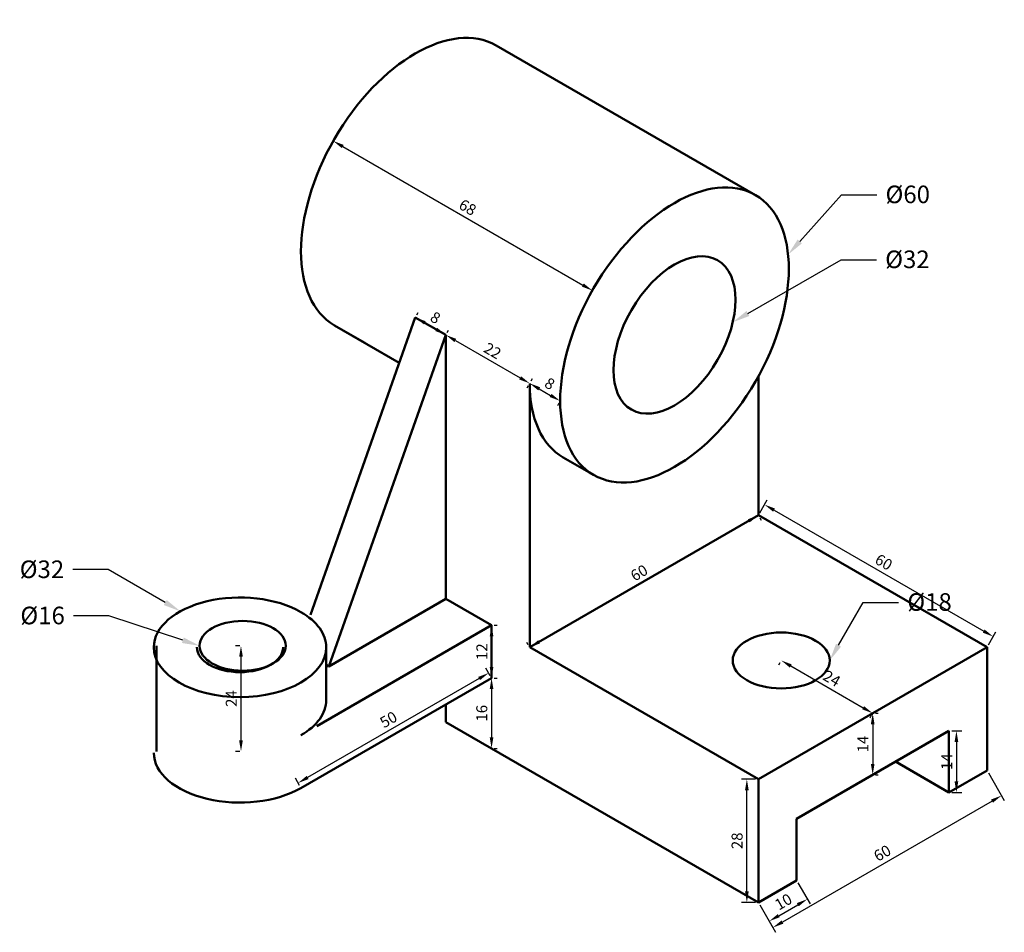
# Model space of a CAD drawing. Units: millimetres. Extents: x 3088 to 3311, y 622 to 830.
import ezdxf
from ezdxf import colors
from ezdxf.entities.mleader import LeaderData, LeaderLine
from ezdxf.math import Vec2, Vec3

# ---------------------------------------------------------------- set-up
doc = ezdxf.new("R2010")
doc.units = ezdxf.units.MM
for name, color, linetype, lineweight in [('M-DIMS', 2, 'Continuous', 25), ('M-OUTL', 7, 'Continuous', 50), ('M-TEXT', 3, 'Continuous', 25)]:
    doc.layers.add(name, color=color, linetype=linetype, lineweight=lineweight)
doc.styles.get("Standard").update_dxf_attribs({"font": 'arial.ttf'})
doc.dimstyles.new('ISO-25', dxfattribs={"dimtxt": 2.5, "dimasz": 2.5, "dimexe": 1.25, "dimexo": 0.625, "dimtad": 1, "dimtxsty": 'Standard', "dimcen": 2.5, "dimadec": 0, "dimazin": 0, "dimtfac": 1, "dimtmove": 0, "dimatfit": 3, "dimfxl": 1, "dimarcsym": 0})

# ---------------------------------------------------------------- blocks, each defined once
blk = doc.blocks.new('*D1')
at = {"layer": 'Defpoints', "color": 0, "transparency": 16777216}
for p in [(3264.1, 633.89), (3255.44, 628.89), (3266.57, 629.62)]:
    blk.add_point(p, dxfattribs=at)
at = {"layer": 'M-DIMS', "color": 0, "lineweight": -2, "transparency": 16777216}
for p, q in [((3264.41, 633.35), (3267.19, 628.53)), ((3255.75, 628.35), (3258.53, 623.53)), ((3260.07, 625.87), (3264.4, 628.37))]:
    blk.add_line(p, q, dxfattribs=at)
at = {"layer": 'M-DIMS', "color": 0, "transparency": 16777216}
for points in [[(3264.19, 628.73), (3264.61, 628.01), (3266.57, 629.62)], [(3259.86, 626.23), (3260.28, 625.51), (3257.91, 624.62)]]:
    blk.add_solid(points, dxfattribs=at)
at = {"layer": 'M-DIMS', "color": 0, "transparency": 16777216, "insert": (3261.29, 628.76), "char_height": 2.5, "attachment_point": 5, "rotation": 30}
blk.add_mtext('10', dxfattribs=at)
blk = doc.blocks.new('*D2')
at = {"layer": 'Defpoints', "color": 0, "transparency": 16777216}
for p in [(3281.42, 671.89), (3281.42, 657.89), (3281.42, 657.89)]:
    blk.add_point(p, dxfattribs=at)
at = {"layer": 'M-DIMS', "color": 0, "lineweight": -2, "transparency": 16777216}
for p, q in [((3282.05, 671.89), (3282.67, 671.89)), ((3281.42, 669.39), (3281.42, 660.39)), ((3282.05, 657.89), (3282.67, 657.89))]:
    blk.add_line(p, q, dxfattribs=at)
at = {"layer": 'M-DIMS', "color": 0, "transparency": 16777216}
for points in [[(3281, 669.39), (3281.84, 669.39), (3281.42, 671.89)], [(3281, 660.39), (3281.84, 660.39), (3281.42, 657.89)]]:
    blk.add_solid(points, dxfattribs=at)
at = {"layer": 'M-DIMS', "color": 0, "transparency": 16777216, "insert": (3279.54, 664.89), "char_height": 2.5, "attachment_point": 5, "rotation": 90}
blk.add_mtext('14', dxfattribs=at)
blk = doc.blocks.new('*D3')
at = {"layer": 'Defpoints', "color": 0, "transparency": 16777216}
for p in [(3307.4, 658.89), (3255.44, 628.89), (3258.74, 623.17)]:
    blk.add_point(p, dxfattribs=at)
at = {"layer": 'M-DIMS', "color": 0, "lineweight": -2, "transparency": 16777216}
for p, q in [((3307.71, 658.35), (3311.33, 652.09)), ((3308.54, 651.92), (3260.91, 624.42)), ((3255.75, 628.35), (3259.37, 622.09))]:
    blk.add_line(p, q, dxfattribs=at)
at = {"layer": 'M-DIMS', "color": 0, "transparency": 16777216}
for points in [[(3308.33, 652.28), (3308.75, 651.56), (3310.7, 653.17)], [(3260.7, 624.78), (3261.12, 624.06), (3258.74, 623.17)]]:
    blk.add_solid(points, dxfattribs=at)
at = {"layer": 'M-DIMS', "color": 0, "transparency": 16777216, "insert": (3283.77, 639.82), "char_height": 2.5, "attachment_point": 5, "rotation": 30}
blk.add_mtext('60', dxfattribs=at)
blk = doc.blocks.new('*D4')
at = {"layer": 'Defpoints', "color": 0, "transparency": 16777216}
for p in [(3252.83, 656.89), (3255.44, 656.89), (3255.44, 628.89)]:
    blk.add_point(p, dxfattribs=at)
at = {"layer": 'M-DIMS', "color": 0, "lineweight": -2, "transparency": 16777216}
for p, q in [((3254.81, 656.89), (3251.58, 656.89)), ((3252.83, 631.39), (3252.83, 654.39)), ((3254.81, 628.89), (3251.58, 628.89))]:
    blk.add_line(p, q, dxfattribs=at)
at = {"layer": 'M-DIMS', "color": 0, "transparency": 16777216}
for points in [[(3252.41, 654.39), (3253.25, 654.39), (3252.83, 656.89)], [(3252.41, 631.39), (3253.25, 631.39), (3252.83, 628.89)]]:
    blk.add_solid(points, dxfattribs=at)
at = {"layer": 'M-DIMS', "color": 0, "transparency": 16777216, "insert": (3250.93, 642.89), "char_height": 2.5, "attachment_point": 5, "rotation": 90}
blk.add_mtext('28', dxfattribs=at)
blk = doc.blocks.new('*D5')
at = {"layer": 'Defpoints', "color": 0, "transparency": 16777216}
for p in [(3194.82, 679.89), (3194.82, 663.89), (3194.82, 663.89)]:
    blk.add_point(p, dxfattribs=at)
at = {"layer": 'M-DIMS', "color": 0, "lineweight": -2, "transparency": 16777216}
for p, q in [((3195.44, 679.89), (3196.07, 679.89)), ((3194.82, 677.39), (3194.82, 666.39)), ((3195.44, 663.89), (3196.07, 663.89))]:
    blk.add_line(p, q, dxfattribs=at)
at = {"layer": 'M-DIMS', "color": 0, "transparency": 16777216}
for points in [[(3194.4, 677.39), (3195.23, 677.39), (3194.82, 679.89)], [(3194.4, 666.39), (3195.23, 666.39), (3194.82, 663.89)]]:
    blk.add_solid(points, dxfattribs=at)
at = {"layer": 'M-DIMS', "color": 0, "transparency": 16777216, "insert": (3192.92, 671.89), "char_height": 2.5, "attachment_point": 5, "rotation": 90}
blk.add_mtext('16', dxfattribs=at)
blk = doc.blocks.new('*D6')
at = {"layer": 'Defpoints', "color": 0, "transparency": 16777216}
for p in [(3194.82, 691.89), (3194.82, 679.89), (3194.82, 679.89)]:
    blk.add_point(p, dxfattribs=at)
at = {"layer": 'M-DIMS', "color": 0, "lineweight": -2, "transparency": 16777216}
for p, q in [((3195.44, 691.89), (3196.07, 691.89)), ((3194.82, 689.39), (3194.82, 682.39)), ((3195.44, 679.89), (3196.07, 679.89))]:
    blk.add_line(p, q, dxfattribs=at)
at = {"layer": 'M-DIMS', "color": 0, "transparency": 16777216}
for points in [[(3194.4, 689.39), (3195.23, 689.39), (3194.82, 691.89)], [(3194.4, 682.39), (3195.23, 682.39), (3194.82, 679.89)]]:
    blk.add_solid(points, dxfattribs=at)
at = {"layer": 'M-DIMS', "color": 0, "transparency": 16777216, "insert": (3192.94, 685.89), "char_height": 2.5, "attachment_point": 5, "rotation": 90}
blk.add_mtext('12', dxfattribs=at)
blk = doc.blocks.new('*D7')
at = {"layer": 'Defpoints', "color": 0, "transparency": 16777216}
for p in [(3255.44, 716.89), (3255.44, 716.89), (3203.48, 686.89)]:
    blk.add_point(p, dxfattribs=at)
at = {"layer": 'M-DIMS', "color": 0, "lineweight": -2, "transparency": 16777216}
for p, q in [((3255.75, 716.35), (3256.06, 715.81)), ((3205.64, 688.14), (3253.27, 715.64)), ((3203.17, 687.43), (3202.85, 687.97))]:
    blk.add_line(p, q, dxfattribs=at)
at = {"layer": 'M-DIMS', "color": 0, "transparency": 16777216}
for points in [[(3253.07, 716), (3253.48, 715.28), (3255.44, 716.89)], [(3205.43, 688.5), (3205.85, 687.78), (3203.48, 686.89)]]:
    blk.add_solid(points, dxfattribs=at)
at = {"layer": 'M-DIMS', "color": 0, "transparency": 16777216, "insert": (3228.51, 703.54), "char_height": 2.5, "attachment_point": 5, "rotation": 30}
blk.add_mtext('60', dxfattribs=at)
blk = doc.blocks.new('*D8')
at = {"layer": 'Defpoints', "color": 0, "transparency": 16777216}
for p in [(3194.82, 679.89), (3150.86, 656.04), (3151.52, 654.89)]:
    blk.add_point(p, dxfattribs=at)
at = {"layer": 'M-DIMS', "color": 0, "lineweight": -2, "transparency": 16777216}
for p, q in [((3194.51, 680.43), (3193.53, 682.12)), ((3191.99, 679.79), (3153.02, 657.29)), ((3151.2, 655.43), (3150.23, 657.12))]:
    blk.add_line(p, q, dxfattribs=at)
at = {"layer": 'M-DIMS', "color": 0, "transparency": 16777216}
for points in [[(3191.78, 680.15), (3192.2, 679.42), (3194.16, 681.04)], [(3152.81, 657.65), (3153.23, 656.92), (3150.86, 656.04)]]:
    blk.add_solid(points, dxfattribs=at)
at = {"layer": 'M-DIMS', "color": 0, "transparency": 16777216, "insert": (3171.56, 670.18), "char_height": 2.5, "attachment_point": 5, "rotation": 30}
blk.add_mtext('50', dxfattribs=at)
blk = doc.blocks.new('*D9')
at = {"layer": 'Defpoints', "color": 0, "transparency": 16777216}
for p in [(3184.43, 757.89), (3203.48, 746.89), (3203.48, 746.89)]:
    blk.add_point(p, dxfattribs=at)
at = {"layer": 'M-DIMS', "color": 0, "lineweight": -2, "transparency": 16777216}
for p, q in [((3184.74, 758.43), (3185.05, 758.97)), ((3186.59, 756.64), (3201.31, 748.14)), ((3203.79, 747.43), (3204.1, 747.97))]:
    blk.add_line(p, q, dxfattribs=at)
at = {"layer": 'M-DIMS', "color": 0, "transparency": 16777216}
for points in [[(3186.8, 757), (3186.38, 756.28), (3184.43, 757.89)], [(3201.52, 748.5), (3201.1, 747.78), (3203.48, 746.89)]]:
    blk.add_solid(points, dxfattribs=at)
at = {"layer": 'M-DIMS', "color": 0, "transparency": 16777216, "insert": (3194.89, 754.02), "char_height": 2.5, "attachment_point": 5, "rotation": 330}
blk.add_mtext('22', dxfattribs=at)
blk = doc.blocks.new('*D10')
at = {"layer": 'Defpoints', "color": 0, "transparency": 16777216}
for p in [(3177.5, 761.89), (3184.43, 757.89), (3184.43, 757.89)]:
    blk.add_point(p, dxfattribs=at)
at = {"layer": 'M-DIMS', "color": 0, "lineweight": -2, "transparency": 16777216}
for p, q in [((3177.81, 762.43), (3178.12, 762.97)), ((3179.66, 760.64), (3182.26, 759.14)), ((3184.74, 758.43), (3185.05, 758.97))]:
    blk.add_line(p, q, dxfattribs=at)
at = {"layer": 'M-DIMS', "color": 0, "transparency": 16777216}
for points in [[(3179.87, 761), (3179.45, 760.28), (3177.5, 761.89)], [(3182.47, 759.5), (3182.05, 758.78), (3184.43, 757.89)]]:
    blk.add_solid(points, dxfattribs=at)
at = {"layer": 'M-DIMS', "color": 0, "transparency": 16777216, "insert": (3181.91, 761.54), "char_height": 2.5, "attachment_point": 5, "rotation": 330}
blk.add_mtext('8', dxfattribs=at)
blk = doc.blocks.new('*D11')
at = {"layer": 'Defpoints', "color": 0, "transparency": 16777216}
for p in [(3298.74, 667.89), (3298.74, 653.89), (3300.45, 653.89)]:
    blk.add_point(p, dxfattribs=at)
at = {"layer": 'M-DIMS', "color": 0, "lineweight": -2, "transparency": 16777216}
for p, q in [((3299.37, 667.89), (3301.7, 667.89)), ((3300.45, 665.39), (3300.45, 656.39)), ((3299.37, 653.89), (3301.7, 653.89))]:
    blk.add_line(p, q, dxfattribs=at)
at = {"layer": 'M-DIMS', "color": 0, "transparency": 16777216}
for points in [[(3300.03, 665.39), (3300.86, 665.39), (3300.45, 667.89)], [(3300.03, 656.39), (3300.86, 656.39), (3300.45, 653.89)]]:
    blk.add_solid(points, dxfattribs=at)
at = {"layer": 'M-DIMS', "color": 0, "transparency": 16777216, "insert": (3298.57, 660.89), "char_height": 2.5, "attachment_point": 5, "rotation": 90}
blk.add_mtext('14', dxfattribs=at)
blk = doc.blocks.new('*D12')
at = {"layer": 'Defpoints', "color": 0, "transparency": 16777216}
for p in [(3138.27, 687.23), (3137.88, 663.23), (3138.27, 663.23)]:
    blk.add_point(p, dxfattribs=at)
at = {"layer": 'M-DIMS', "color": 0, "lineweight": -2, "transparency": 16777216}
for p, q in [((3137.64, 687.23), (3136.63, 687.23)), ((3137.88, 684.73), (3137.88, 665.73)), ((3137.64, 663.23), (3136.63, 663.23))]:
    blk.add_line(p, q, dxfattribs=at)
at = {"layer": 'M-DIMS', "color": 0, "transparency": 16777216}
for points in [[(3137.46, 684.73), (3138.3, 684.73), (3137.88, 687.23)], [(3137.46, 665.73), (3138.3, 665.73), (3137.88, 663.23)]]:
    blk.add_solid(points, dxfattribs=at)
at = {"layer": 'M-DIMS', "color": 0, "transparency": 16777216, "insert": (3136, 675.23), "char_height": 2.5, "attachment_point": 5, "rotation": 90}
blk.add_mtext('24', dxfattribs=at)
blk = doc.blocks.new('*D13')
at = {"layer": 'Defpoints', "color": 0, "transparency": 16777216}
for p in [(3159.13, 802.5), (3217.72, 767.99), (3218.02, 768.5)]:
    blk.add_point(p, dxfattribs=at)
at = {"layer": 'M-DIMS', "color": 0, "lineweight": -2, "transparency": 16777216}
for p, q in [((3158.81, 801.96), (3158.21, 800.91)), ((3161, 800.74), (3215.56, 769.24)), ((3217.7, 767.96), (3217.1, 766.91))]:
    blk.add_line(p, q, dxfattribs=at)
at = {"layer": 'M-DIMS', "color": 0, "transparency": 16777216}
for points in [[(3161.21, 801.1), (3160.79, 800.38), (3158.83, 801.99)], [(3215.77, 769.6), (3215.35, 768.88), (3217.72, 767.99)]]:
    blk.add_solid(points, dxfattribs=at)
at = {"layer": 'M-DIMS', "color": 0, "transparency": 16777216, "insert": (3189.23, 786.63), "char_height": 2.5, "attachment_point": 5, "rotation": 330}
blk.add_mtext('68', dxfattribs=at)
blk = doc.blocks.new('*D14')
at = {"layer": 'Defpoints', "color": 0, "transparency": 16777216}
for p in [(3203.48, 746.89), (3210.41, 742.89), (3210.41, 742.89)]:
    blk.add_point(p, dxfattribs=at)
at = {"layer": 'M-DIMS', "color": 0, "lineweight": -2, "transparency": 16777216}
for p, q in [((3203.17, 746.35), (3202.85, 745.81)), ((3205.64, 745.64), (3208.24, 744.14)), ((3210.09, 742.35), (3209.78, 741.81))]:
    blk.add_line(p, q, dxfattribs=at)
at = {"layer": 'M-DIMS', "color": 0, "transparency": 16777216}
for points in [[(3205.85, 746), (3205.43, 745.28), (3203.48, 746.89)], [(3208.45, 744.5), (3208.03, 743.78), (3210.41, 742.89)]]:
    blk.add_solid(points, dxfattribs=at)
at = {"layer": 'M-DIMS', "color": 0, "transparency": 16777216, "insert": (3207.89, 746.54), "char_height": 2.5, "attachment_point": 5, "rotation": 330}
blk.add_mtext('8', dxfattribs=at)
blk = doc.blocks.new('*D15')
at = {"layer": 'Defpoints', "color": 0, "transparency": 16777216}
for p in [(3260.64, 683.89), (3281.42, 671.89), (3281.42, 671.89)]:
    blk.add_point(p, dxfattribs=at)
at = {"layer": 'M-DIMS', "color": 0, "lineweight": -2, "transparency": 16777216}
for p, q in [((3260.32, 683.35), (3260.01, 682.81)), ((3262.8, 682.64), (3279.26, 673.14)), ((3281.11, 671.35), (3280.8, 670.81))]:
    blk.add_line(p, q, dxfattribs=at)
at = {"layer": 'M-DIMS', "color": 0, "transparency": 16777216}
for points in [[(3263.01, 683), (3262.59, 682.28), (3260.64, 683.89)], [(3279.46, 673.5), (3279.05, 672.78), (3281.42, 671.89)]]:
    blk.add_solid(points, dxfattribs=at)
at = {"layer": 'M-DIMS', "color": 0, "transparency": 16777216, "insert": (3271.97, 679.52), "char_height": 2.5, "attachment_point": 5, "rotation": 330}
blk.add_mtext('24', dxfattribs=at)
blk = doc.blocks.new('*D16')
at = {"layer": 'Defpoints', "color": 0, "transparency": 16777216}
for p in [(3255.44, 716.89), (3308.81, 689.32), (3307.4, 686.89)]:
    blk.add_point(p, dxfattribs=at)
at = {"layer": 'M-DIMS', "color": 0, "lineweight": -2, "transparency": 16777216}
for p, q in [((3255.75, 717.43), (3257.47, 720.41)), ((3259.01, 718.07), (3306.64, 690.57)), ((3307.71, 687.43), (3309.43, 690.41))]:
    blk.add_line(p, q, dxfattribs=at)
at = {"layer": 'M-DIMS', "color": 0, "transparency": 16777216}
for points in [[(3259.22, 718.43), (3258.8, 717.71), (3256.84, 719.32)], [(3306.85, 690.93), (3306.43, 690.21), (3308.81, 689.32)]]:
    blk.add_solid(points, dxfattribs=at)
at = {"layer": 'M-DIMS', "color": 0, "transparency": 16777216, "insert": (3283.78, 705.97), "char_height": 2.5, "attachment_point": 5, "rotation": 330}
blk.add_mtext('60', dxfattribs=at)

msp = doc.modelspace()

# ---------------------------------------------------------------- linework, layer by layer
at = {"layer": 'M-OUTL'}
for p, q in [((3254.758, 789.71), (3195.869, 823.71)), ((3177.497, 761.89), (3153.645, 694.239)), ((3184.426, 757.89), (3177.497, 761.89)), ((3159.126, 760.07), (3166.054, 756.07)), ((3173.857, 751.565), (3159.126, 760.07)), ((3184.426, 757.89), (3157.863, 682.554)), ((3184.426, 757.89), (3184.426, 697.89)), ((3255.44, 748.494), (3255.44, 716.89)), ((3203.478, 686.89), (3203.478, 746.89)), ((3218.016, 726.07), (3211.088, 730.07)), ((3255.44, 716.89), (3203.478, 686.89)), ((3307.401, 686.89), (3255.44, 716.89)), ((3118.671, 687.226), (3118.671, 663.226)), ((3157.256, 674.89), (3157.256, 686.89)), ((3203.478, 686.89), (3255.44, 656.89)), ((3255.44, 656.89), (3307.401, 686.89)), ((3307.401, 686.89), (3307.401, 658.89)), ((3157.863, 682.554), (3157.256, 682.904)), ((3184.426, 673.89), (3184.426, 669.89)), ((3255.44, 628.89), (3184.426, 669.89)), ((3298.741, 667.89), (3264.1, 647.89)), ((3298.741, 667.89), (3298.741, 653.89)), ((3298.741, 653.89), (3286.617, 660.89)), ((3307.401, 658.89), (3298.741, 653.89)), ((3255.44, 628.89), (3255.44, 656.89)), ((3264.1, 647.89), (3264.1, 633.89)), ((3264.1, 633.89), (3255.44, 628.89))]:
    msp.add_line(p, q, dxfattribs=at)
for points in [[(3157.863, 682.554), (3184.426, 697.89), (3194.818, 691.89)], [(3155.138, 668.981), (3194.818, 691.89), (3194.818, 679.89), (3151.517, 654.89)]]:
    msp.add_lwpolyline(points, dxfattribs=at)
for centre, major_axis, start_param, end_param in [((3177.497, 791.89), (-18.371, -31.82), 3.1415927, 6.2831853), ((3229.459, 761.89), (18.371, 31.82), 2.3561945, 3.1415927), ((3137.66, 686.89), (19.596, 0), 0.7853982, 3.1415927), ((3137.66, 686.89), (19.596, 0), 0, 0.7853982), ((3137.66, 686.89), (19.596, 0), 3.1415927, 6.2831853), ((3137.66, 686.89), (9.798, 0), 3.1415927, 6.2831853), ((3137.66, 674.89), (19.596, 0), 5.4977871, 6.2831853), ((3137.66, 662.89), (19.596, 0), 3.1415927, 5.4977871)]:
    msp.add_ellipse(centre, major_axis=major_axis, ratio=0.5773503, start_param=start_param, end_param=end_param, dxfattribs=at)
for centre, major_axis in [((3236.387, 757.89), (-18.371, -31.82)), ((3236.387, 757.89), (-9.798, -16.971)), ((3138.267, 687.226), (-9.798, 0)), ((3260.636, 683.89), (-11.023, 0))]:
    msp.add_ellipse(centre, major_axis=major_axis, ratio=0.5773503, dxfattribs=at)

# ---------------------------------------------------------------- dimensions: what is measured, and where the dimension line sits
at = {"layer": 'M-DIMS'}
for p1, p2, distance, picture, middle in [((3159.126, 802.497), (3218.016, 768.497), -0.588, '*D13', (3189.228, 786.635)), ((3177.497, 761.89), (3184.426, 757.89), 0, '*D10', (3181.912, 761.537)), ((3184.426, 757.89), (3203.478, 746.89), 0, '*D9', (3194.892, 754.018)), ((3203.478, 746.89), (3210.406, 742.89), 0, '*D14', (3207.893, 746.537)), ((3255.44, 716.89), (3307.401, 686.89), 2.81, '*D16', (3283.776, 705.97)), ((3203.478, 686.89), (3255.44, 716.89), 0, '*D7', (3228.508, 703.537)), ((3260.636, 683.89), (3281.42, 671.89), 0, '*D15', (3271.968, 679.518)), ((3194.818, 679.89), (3151.517, 654.89), -1.322, '*D8', (3171.556, 670.182)), ((3281.42, 671.89), (3281.42, 657.89), 0, '*D2', (3279.54, 664.89)), ((3307.401, 658.89), (3255.44, 628.89), 6.605, '*D3', (3283.772, 639.817)), ((3255.44, 628.89), (3255.44, 656.89), 2.608, '*D4', (3250.93, 642.89)), ((3255.44, 628.89), (3264.1, 633.89), -4.934, '*D1', (3261.286, 628.764))]:
    dim = msp.add_aligned_dim(p1=p1, p2=p2, distance=distance, dimstyle='ISO-25', override={"dimclrd": 0, "dimclre": 0, "dimclrt": 0}, dxfattribs=at)
    dim.commit()
    dim.dimension.update_dxf_attribs({"geometry": picture, "text_midpoint": middle})
for base, p1, p2, picture, middle in [((3194.818, 679.89), (3194.818, 691.89), (3194.818, 679.89), '*D6', (3192.938, 685.89)), ((3137.878, 663.226), (3138.267, 687.226), (3138.267, 663.226), '*D12', (3135.998, 675.226)), ((3194.818, 663.89), (3194.818, 679.89), (3194.818, 663.89), '*D5', (3192.916, 671.89)), ((3300.448, 653.89), (3298.741, 667.89), (3298.741, 653.89), '*D11', (3298.568, 660.89))]:
    dim = msp.add_linear_dim(base=base, p1=p1, p2=p2, angle=90, dimstyle='ISO-25', override={"dimclrd": 0, "dimclre": 0, "dimclrt": 0}, dxfattribs=at)
    dim.commit()
    dim.dimension.update_dxf_attribs({"geometry": picture, "text_midpoint": middle})

# ---------------------------------------------------------------- leaders
at = {"layer": 'M-TEXT'}
ml = msp.add_multileader_mtext('Standard', dxfattribs=at)
ml.set_content('%%C60', color=256)
ml.set_leader_properties()
ml.build(insert=Vec2(0, 0))
ctx = ml.context
ctx.base_point, ctx.plane_origin = Vec3(3282.335, 789.774), Vec3(3262.203, 776.173)
notes = []
notes.append((ctx, [(0, (1, 1, 0), (3274.335, 789.774), (1, 0), 8, [(0, [(3262.203, 776.173)], 0, [])])]))
ctx.mtext.insert, ctx.mtext.flow_direction = Vec3(3284.335, 791.854), 5
ml = msp.add_multileader_mtext('Standard', dxfattribs=at)
ml.set_content('%%C32', color=256)
ml.set_leader_properties()
ml.build(insert=Vec2(0, 0))
ctx = ml.context
ctx.base_point, ctx.plane_origin = Vec3(3282.26, 775.005), Vec3(3249.619, 760.778)
notes.append((ctx, [(0, (1, 1, 0), (3274.26, 775.005), (1, 0), 8, [(0, [(3249.619, 760.778)], 0, [])])]))
ctx.mtext.insert, ctx.mtext.flow_direction = Vec3(3284.26, 777.085), 5
ml = msp.add_multileader_mtext('Standard', dxfattribs=at)
ml.set_content('%%C32', color=256)
ml.set_leader_properties()
ml.build(insert=Vec2(0, 0))
ctx = ml.context
ctx.base_point, ctx.plane_origin = Vec3(3085.662, 704.542), Vec3(3124.128, 695.059)
ctx.text_align_type = 2
notes.append((ctx, [(0, (1, 1, 0), (3107.703, 704.542), (-1, 0), 8, [(0, [(3124.128, 695.059)], 0, [])])]))
ctx.mtext.insert, ctx.mtext.alignment, ctx.mtext.flow_direction = Vec3(3097.703, 706.622), 3, 5
ml = msp.add_multileader_mtext('Standard', dxfattribs=at)
ml.set_content('%%C18', color=256)
ml.set_leader_properties()
ml.build(insert=Vec2(0, 0))
ctx = ml.context
ctx.base_point, ctx.plane_origin = Vec3(3287.287, 697.104), Vec3(3271.659, 683.89)
notes.append((ctx, [(0, (1, 1, 0), (3279.287, 697.104), (1, 0), 8, [(0, [(3271.659, 683.89)], 0, [])])]))
ctx.mtext.insert, ctx.mtext.flow_direction = Vec3(3289.287, 699.184), 5
ml = msp.add_multileader_mtext('Standard', dxfattribs=at)
ml.set_content('%%C16', color=256)
ml.set_leader_properties()
ml.build(insert=Vec2(0, 0))
ctx = ml.context
ctx.base_point, ctx.plane_origin = Vec3(3085.774, 694.034), Vec3(3128.469, 687.226)
ctx.text_align_type = 2
notes.append((ctx, [(0, (1, 1, 0), (3107.853, 694.034), (-1, 0), 8, [(0, [(3128.469, 687.226)], 0, [])])]))
ctx.mtext.insert, ctx.mtext.alignment, ctx.mtext.flow_direction = Vec3(3097.853, 696.114), 3, 5
for ctx, leaders in notes:
    for number, flags, end, landing, length, lines in leaders:
        leader = LeaderData()
        leader.index, (leader.has_last_leader_line, leader.has_dogleg_vector, leader.attachment_direction) = number, flags
        leader.last_leader_point, leader.dogleg_vector, leader.dogleg_length = Vec3(end), Vec3(landing), length
        for number, points, colour, breaks in lines:
            line = LeaderLine()
            line.index, line.vertices, line.color, line.breaks = number, Vec3.list(points), colors.encode_raw_color(colour), breaks
            leader.lines.append(line)
        ctx.leaders.append(leader)

doc.saveas('drawing.dxf')
